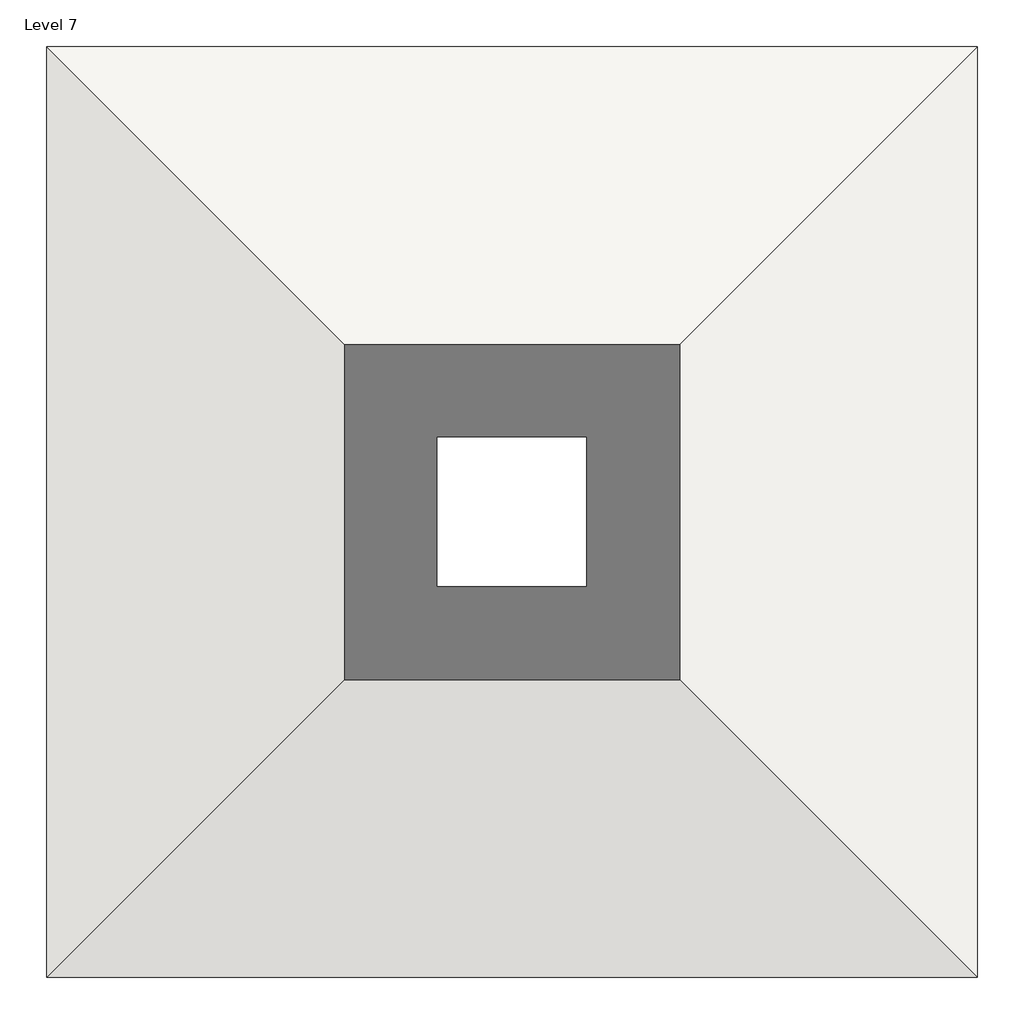
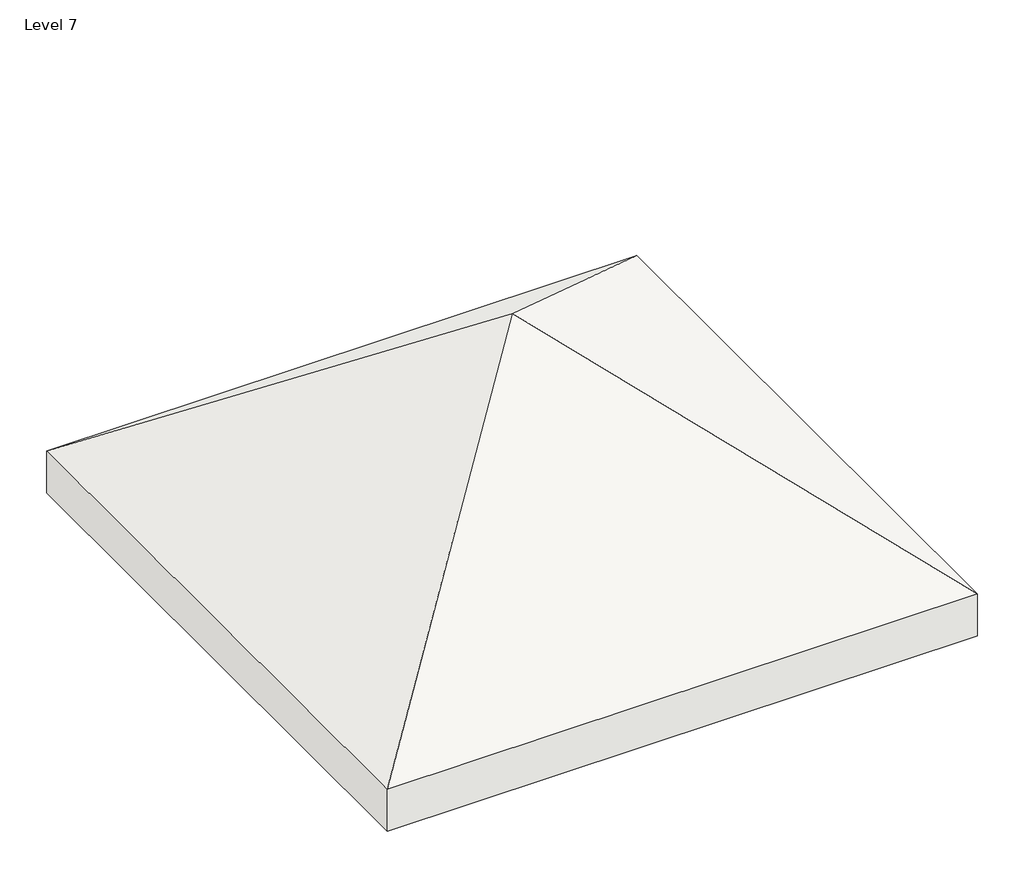
# One storey: 1 roof.
"""IFC4 building model written with IfcOpenShell, lengths in millimetres."""

from ifc_helpers import new_model, si_unit, origin, place, context, project, spatial, faceted_brep, element, save

model = new_model("IFC4")

# Units and contexts
model_context = context("Model", 3, world=origin())
ifc_project = project(units=[si_unit("LENGTHUNIT", "METRE", prefix="MILLI")], contexts=[model_context])

# Site, building, storey
site = spatial("IfcSite", under=ifc_project)
building = spatial("IfcBuilding", under=site)
storey = spatial("IfcBuildingStorey", under=building, Name="Level 7", Elevation=9601.2)

# Roof
placement = place(None, origin())
element("IfcRoof", 1, ObjectType="Generic - 9\"", at=placement, inside=storey, context=model_context, shape_type="Brep", body=[
    faceted_brep([(-5802.6592501, 12895.113343, 9601.2), (-7707.6592501, 10990.113343, 11029.95), (-9612.6592501, 12895.113343, 9601.2), (-9612.6592501, 9085.113343, 9601.2), (-5802.6592501, 9085.113343, 9601.2), (-5802.6592501, 12895.113343, 9886.95), (-9612.6592501, 12895.113343, 9886.95), (-7707.6592501, 10990.113343, 11315.7), (-9612.6592501, 9085.113343, 9886.95), (-5802.6592501, 9085.113343, 9886.95)], [[[0, 1, 2]], [[2, 1, 3]], [[3, 1, 4]], [[1, 0, 4]], [[5, 6, 7]], [[6, 8, 7]], [[8, 9, 7]], [[5, 7, 9]], [[2, 6, 5, 0]], [[3, 8, 6, 2]], [[4, 9, 8, 3]], [[0, 5, 9, 4]]]),
])

save(model, "model.ifc")

# Revit data of these elements
# Type "Generic - 9\""
#   Assembly Code = "B1020"
#   Layers, outside or top first: 0' - 9" no material (function 1)
# Element 1 (IfcRoof, "Generic - 9\"")
#   built-in parameter 1001705 = 37.125 (stored number, unit not read)
#   built-in parameter 1001710 = 33615
#   Phase Created = New Construction
#   Materials on its faces: "Default Roof"
# Materials
#   "Default Roof": colour RGB 88 101 114, transparency 0
